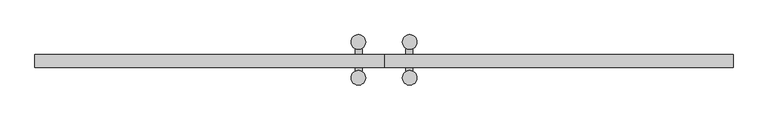
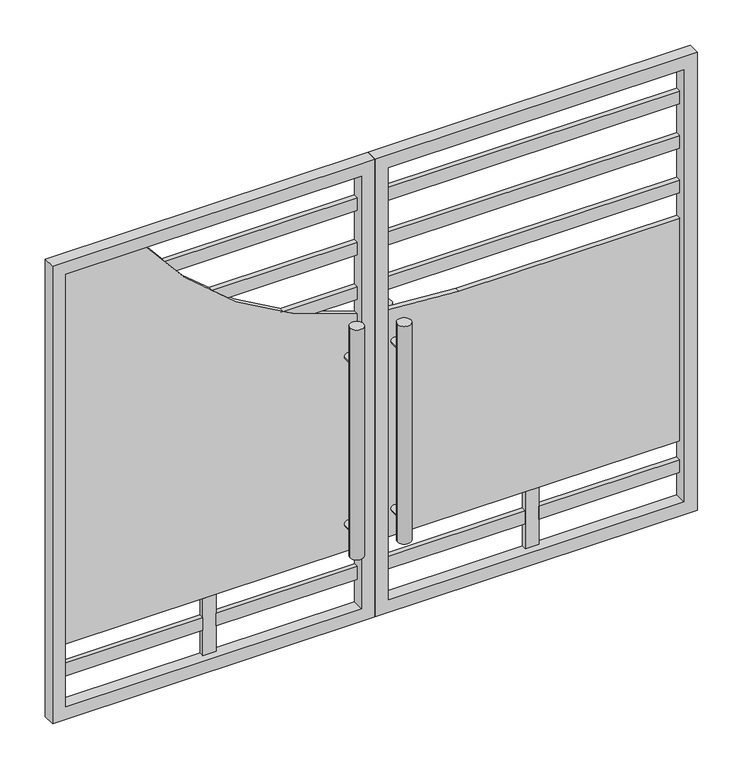
"""IFC4 building model written with IfcOpenShell, lengths in millimetres: proxy geometry."""

from ifc_helpers import new_model, si_unit, point, frame, frame_2d, origin, place, context, project, spatial, polyline, circle_curve, trimmed, segment, composite_curve, outline, extrude, source, transform, mapped, element, save


def generic_models_113f6068(model_context):
    return source(origin(), model_context, "Body", "SweptSolid", [
        extrude(outline(polyline([(0.0, -1219.2), (0.0, 0.0), (1828.8, 0.0), (1828.8, -1219.2), (0.0, -1219.2)]), holes=[polyline([(50.8, -1168.4), (1778.0, -1168.4), (1778.0, -50.8), (50.8, -50.8), (50.8, -1168.4)])]), frame((0.0, -46.0617726, 0.0), z_axis=(0.0, 1.0, 0.0), x_axis=(0.0, 0.0, 1.0)), (0.0, 0.0, 1.0), 46.0617726),
        extrude(outline(polyline([(0.0, 1219.2), (1828.8, 1219.2), (1828.8, 0.0), (0.0, 0.0), (0.0, 1219.2)]), holes=[polyline([(50.8, 1168.4), (50.8, 50.8), (1778.0, 50.8), (1778.0, 1168.4), (50.8, 1168.4)])]), frame((0.0, -46.0617726, 0.0), z_axis=(0.0, 1.0, 0.0), x_axis=(0.0, 0.0, 1.0)), (0.0, 0.0, 1.0), 46.0617726),
        extrude(outline(composite_curve([segment(polyline([(1778.0, -1168.4), (279.4, -1168.4), (279.4, -50.8), (1212.1744192, -50.8)]), True, "CONTINUOUS"), segment(trimmed(circle_curve(frame_2d((2582.6324877, 299.8877691)), 1414.6155764), [point((1212.1744192, -50.8))], [point((1778.0, -863.6))], True, "CARTESIAN"), True, "CONTINUOUS"), segment(polyline([(1778.0, -863.6), (1778.0, -1168.4)]), True, "CONTINUOUS")], self_intersect=False)), frame((0.0, -19.05, 0.0), z_axis=(0.0, 1.0, 0.0), x_axis=(0.0, 0.0, 1.0)), (0.0, 0.0, 1.0), 19.05),
        extrude(outline(composite_curve([segment(polyline([(279.4, 1168.4), (1168.4, 1168.4), (1168.4, 332.8073642)]), True, "CONTINUOUS"), segment(trimmed(circle_curve(frame_2d((2582.6324877, 299.8877691)), 1414.6155764), [point((1168.4, 332.8073642))], [point((1190.1194672, 50.8))], True, "CARTESIAN"), True, "CONTINUOUS"), segment(polyline([(1190.1194672, 50.8), (279.4, 50.8), (279.4, 1168.4)]), True, "CONTINUOUS")], self_intersect=False)), frame((0.0, -19.05, 0.0), z_axis=(0.0, 1.0, 0.0), x_axis=(0.0, 0.0, 1.0)), (0.0, 0.0, 1.0), 19.05),
        extrude(outline(composite_curve([segment(polyline([(1676.4, -50.8), (1676.4, -786.3350015)]), True, "CONTINUOUS"), segment(trimmed(circle_curve(frame_2d((2582.6324877, 299.8877691)), 1414.6155764), [point((1676.4, -786.3350015))], [point((1625.6, -741.8540639))], False, "CARTESIAN"), True, "CONTINUOUS"), segment(polyline([(1625.6, -741.8540639), (1625.6, -50.8), (1676.4, -50.8)]), True, "CONTINUOUS")], self_intersect=False)), frame((0.0, -19.05, 0.0), z_axis=(0.0, 1.0, 0.0), x_axis=(0.0, 0.0, 1.0)), (0.0, 0.0, 1.0), 19.05),
        extrude(outline(polyline([(1171.575, -19.05), (50.8, -19.05), (50.8, 0.0), (1171.575, 0.0), (1171.575, -19.05)])), frame((0.0, 0.0, 1625.6), z_axis=(0.0, 0.0, 1.0), x_axis=(1.0, 0.0, 0.0)), (0.0, 0.0, 1.0), 50.8),
        extrude(outline(composite_curve([segment(polyline([(1498.6, -50.8), (1498.6, -608.963591)]), True, "CONTINUOUS"), segment(trimmed(circle_curve(frame_2d((2582.6324877, 299.8877691)), 1414.6155764), [point((1498.6, -608.963591))], [point((1447.8, -544.6786605))], False, "CARTESIAN"), True, "CONTINUOUS"), segment(polyline([(1447.8, -544.6786605), (1447.8, -50.8), (1498.6, -50.8)]), True, "CONTINUOUS")], self_intersect=False)), frame((0.0, -19.05, 0.0), z_axis=(0.0, 1.0, 0.0), x_axis=(0.0, 0.0, 1.0)), (0.0, 0.0, 1.0), 19.05),
        extrude(outline(polyline([(1171.575, -19.05), (50.8, -19.05), (50.8, 0.0), (1171.575, 0.0), (1171.575, -19.05)])), frame((0.0, 0.0, 1447.8), z_axis=(0.0, 0.0, 1.0), x_axis=(1.0, 0.0, 0.0)), (0.0, 0.0, 1.0), 50.8),
        extrude(outline(composite_curve([segment(polyline([(1320.8, -50.8), (1320.8, -339.5776342)]), True, "CONTINUOUS"), segment(trimmed(circle_curve(frame_2d((2582.6324877, 299.8877691)), 1414.6155764), [point((1320.8, -339.5776342))], [point((1270.0, -227.4955652))], False, "CARTESIAN"), True, "CONTINUOUS"), segment(polyline([(1270.0, -227.4955652), (1270.0, -50.8), (1320.8, -50.8)]), True, "CONTINUOUS")], self_intersect=False)), frame((0.0, -19.05, 0.0), z_axis=(0.0, 1.0, 0.0), x_axis=(0.0, 0.0, 1.0)), (0.0, 0.0, 1.0), 19.05),
        extrude(outline(polyline([(1171.575, -19.05), (50.8, -19.05), (50.8, 0.0), (1171.575, 0.0), (1171.575, -19.05)])), frame((0.0, 0.0, 1270.0), z_axis=(0.0, 0.0, 1.0), x_axis=(1.0, 0.0, 0.0)), (0.0, 0.0, 1.0), 50.8),
        extrude(outline(polyline([(-635.0, -19.05), (-1168.4, -19.05), (-1168.4, 0.0), (-635.0, 0.0), (-635.0, -19.05)])), frame((0.0, 0.0, 152.4), z_axis=(0.0, 0.0, 1.0), x_axis=(1.0, 0.0, 0.0)), (0.0, 0.0, 1.0), 50.8),
        extrude(outline(polyline([(-50.8, -19.05), (-584.2, -19.05), (-584.2, 0.0), (-50.8, 0.0), (-50.8, -19.05)])), frame((0.0, 0.0, 152.4), z_axis=(0.0, 0.0, 1.0), x_axis=(1.0, 0.0, 0.0)), (0.0, 0.0, 1.0), 50.8),
        extrude(outline(polyline([(1168.4, -19.05), (635.0, -19.05), (635.0, 0.0), (1168.4, 0.0), (1168.4, -19.05)])), frame((0.0, 0.0, 152.4), z_axis=(0.0, 0.0, 1.0), x_axis=(1.0, 0.0, 0.0)), (0.0, 0.0, 1.0), 50.8),
        extrude(outline(polyline([(584.2, -19.05), (50.8, -19.05), (50.8, 0.0), (584.2, 0.0), (584.2, -19.05)])), frame((0.0, 0.0, 152.4), z_axis=(0.0, 0.0, 1.0), x_axis=(1.0, 0.0, 0.0)), (0.0, 0.0, 1.0), 50.8),
        extrude(outline(polyline([(-584.2, -19.05), (-635.0, -19.05), (-635.0, 0.0), (-584.2, 0.0), (-584.2, -19.05)])), frame((0.0, 0.0, 50.8), z_axis=(0.0, 0.0, 1.0), x_axis=(1.0, 0.0, 0.0)), (0.0, 0.0, 1.0), 228.6),
        extrude(outline(polyline([(635.0, -19.05), (584.2, -19.05), (584.2, 0.0), (635.0, 0.0), (635.0, -19.05)])), frame((0.0, 0.0, 50.8), z_axis=(0.0, 0.0, 1.0), x_axis=(1.0, 0.0, 0.0)), (0.0, 0.0, 1.0), 228.6),
        extrude(outline(composite_curve([segment(trimmed(circle_curve(frame_2d((-89.7949058, 43.7785099)), 25.4), [point((-64.3949058, 43.7785099))], [point((-115.1949058, 43.7785099))], False, "CARTESIAN"), True, "CONTINUOUS"), segment(trimmed(circle_curve(frame_2d((-89.7949058, 43.7785099)), 25.4), [point((-115.1949058, 43.7785099))], [point((-64.3949058, 43.7785099))], False, "CARTESIAN"), True, "CONTINUOUS")], self_intersect=False)), frame((0.0, 0.0, 279.4), z_axis=(0.0, 0.0, 1.0), x_axis=(1.0, 0.0, 0.0)), (0.0, 0.0, 1.0), 889.0),
        extrude(outline(composite_curve([segment(trimmed(circle_curve(frame_2d((89.7949058, 43.7785099)), 25.4), [point((64.3949058, 43.7785099))], [point((115.1949058, 43.7785099))], False, "CARTESIAN"), True, "CONTINUOUS"), segment(trimmed(circle_curve(frame_2d((89.7949058, 43.7785099)), 25.4), [point((115.1949058, 43.7785099))], [point((64.3949058, 43.7785099))], False, "CARTESIAN"), True, "CONTINUOUS")], self_intersect=False)), frame((0.0, 0.0, 279.4), z_axis=(0.0, 0.0, 1.0), x_axis=(1.0, 0.0, 0.0)), (0.0, 0.0, 1.0), 889.0),
        extrude(outline(composite_curve([segment(trimmed(circle_curve(frame_2d((-89.7949058, -81.8785099)), 25.4), [point((-64.3949058, -81.8785099))], [point((-115.1949058, -81.8785099))], False, "CARTESIAN"), True, "CONTINUOUS"), segment(trimmed(circle_curve(frame_2d((-89.7949058, -81.8785099)), 25.4), [point((-115.1949058, -81.8785099))], [point((-64.3949058, -81.8785099))], False, "CARTESIAN"), True, "CONTINUOUS")], self_intersect=False)), frame((0.0, 0.0, 298.8472671), z_axis=(0.0, 0.0, 1.0), x_axis=(1.0, 0.0, 0.0)), (0.0, 0.0, 1.0), 917.3073645),
        extrude(outline(composite_curve([segment(trimmed(circle_curve(frame_2d((89.7949058, -81.8785099)), 25.4), [point((64.3949058, -81.8785099))], [point((115.1949058, -81.8785099))], False, "CARTESIAN"), True, "CONTINUOUS"), segment(trimmed(circle_curve(frame_2d((89.7949058, -81.8785099)), 25.4), [point((115.1949058, -81.8785099))], [point((64.3949058, -81.8785099))], False, "CARTESIAN"), True, "CONTINUOUS")], self_intersect=False)), frame((0.0, 0.0, 298.8472671), z_axis=(0.0, 0.0, 1.0), x_axis=(1.0, 0.0, 0.0)), (0.0, 0.0, 1.0), 869.5527329),
        extrude(outline(composite_curve([segment(trimmed(circle_curve(frame_2d((1058.3458504, 88.119132)), 12.7), [point((1058.3458504, 75.419132))], [point((1058.3458504, 100.819132))], False, "CARTESIAN"), True, "CONTINUOUS"), segment(trimmed(circle_curve(frame_2d((1058.3458504, 88.119132)), 12.7), [point((1058.3458504, 100.819132))], [point((1058.3458504, 75.419132))], False, "CARTESIAN"), True, "CONTINUOUS")], self_intersect=False)), frame((0.0, -57.15, 0.0), z_axis=(0.0, 1.0, 0.0), x_axis=(0.0, 0.0, 1.0)), (0.0, 0.0, 1.0), 76.6172039),
        extrude(outline(composite_curve([segment(trimmed(circle_curve(frame_2d((389.4541496, 88.119132)), 12.7), [point((389.4541496, 75.419132))], [point((389.4541496, 100.819132))], False, "CARTESIAN"), True, "CONTINUOUS"), segment(trimmed(circle_curve(frame_2d((389.4541496, 88.119132)), 12.7), [point((389.4541496, 100.819132))], [point((389.4541496, 75.419132))], False, "CARTESIAN"), True, "CONTINUOUS")], self_intersect=False)), frame((0.0, -57.15, 0.0), z_axis=(0.0, 1.0, 0.0), x_axis=(0.0, 0.0, 1.0)), (0.0, 0.0, 1.0), 76.7981605),
        extrude(outline(composite_curve([segment(trimmed(circle_curve(frame_2d((1058.3458504, -88.119132)), 12.7), [point((1058.3458504, -75.419132))], [point((1058.3458504, -100.819132))], False, "CARTESIAN"), True, "CONTINUOUS"), segment(trimmed(circle_curve(frame_2d((1058.3458504, -88.119132)), 12.7), [point((1058.3458504, -100.819132))], [point((1058.3458504, -75.419132))], False, "CARTESIAN"), True, "CONTINUOUS")], self_intersect=False)), frame((0.0, -57.15, 0.0), z_axis=(0.0, 1.0, 0.0), x_axis=(0.0, 0.0, 1.0)), (0.0, 0.0, 1.0), 76.6172039),
        extrude(outline(composite_curve([segment(trimmed(circle_curve(frame_2d((389.4541496, -88.119132)), 12.7), [point((389.4541496, -75.419132))], [point((389.4541496, -100.819132))], False, "CARTESIAN"), True, "CONTINUOUS"), segment(trimmed(circle_curve(frame_2d((389.4541496, -88.119132)), 12.7), [point((389.4541496, -100.819132))], [point((389.4541496, -75.419132))], False, "CARTESIAN"), True, "CONTINUOUS")], self_intersect=False)), frame((0.0, -57.15, 0.0), z_axis=(0.0, 1.0, 0.0), x_axis=(0.0, 0.0, 1.0)), (0.0, 0.0, 1.0), 76.7981605),
    ])


if __name__ == "__main__":
    model = new_model("IFC4")
    model_context = context("Model", 3, world=origin())
    ifc_project = project(units=[si_unit("LENGTHUNIT", "METRE", prefix="MILLI")], contexts=[model_context])
    site = spatial("IfcSite", under=ifc_project)
    building = spatial("IfcBuilding", under=site)
    placement = place(None, origin())
    generic_models_shape = generic_models_113f6068(model_context)
    element("IfcBuildingElementProxy", 1, Name="Generic Models", at=placement, inside=building, context=model_context, shape_type="MappedRepresentation", body=[
        mapped(generic_models_shape, transform((0.0, 0.0, 0.0), x_axis=(1.0, 0.0, 0.0), y_axis=(0.0, 1.0, 0.0), z_axis=(0.0, 0.0, 1.0))),
    ])
    save(model, "model.ifc")

# Revit data of these elements
# Type
#   sheet = none
#   pipe = none
#   handal = none
#   faram = none
#   Default Elevation = 0
# Element 1 (IfcBuildingElementProxy)
#   Materials on its faces: "Earth"
# Materials
#   "Earth": class "Generic", colour RGB 97 75 62, transparency 0, Description = "Soil", Cost = 0
